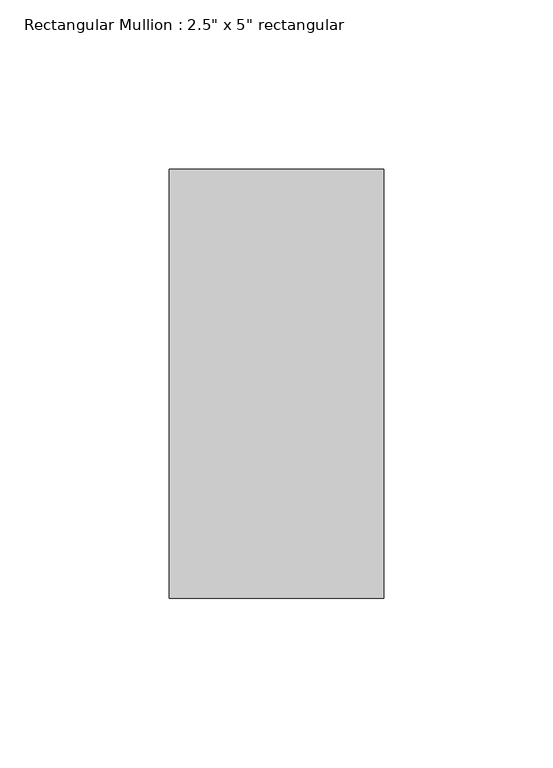
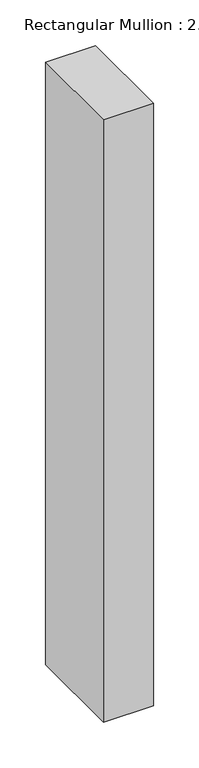
"""IFC4 building model written with IfcOpenShell, lengths in millimetres: member geometry."""

from ifc_helpers import new_model, si_unit, frame, origin, place, context, project, spatial, polyline, outline, extrude, source, transform, mapped, element, save


def member_6e893292(model_context):
    return source(origin(), model_context, "Body", "SweptSolid", [
        extrude(outline(polyline([(31.75, 63.5), (31.75, -63.5), (-31.75, -63.5), (-31.75, 63.5), (31.75, 63.5)])), frame((0.0, 0.0, -806.1882113), z_axis=(0.0, 0.0, 1.0), x_axis=(1.0, 0.0, 0.0)), (0.0, 0.0, 1.0), 806.1882113),
    ])


if __name__ == "__main__":
    model = new_model("IFC4")
    model_context = context("Model", 3, world=origin())
    ifc_project = project(units=[si_unit("LENGTHUNIT", "METRE", prefix="MILLI")], contexts=[model_context])
    site = spatial("IfcSite", under=ifc_project)
    building = spatial("IfcBuilding", under=site)
    placement = place(None, origin())
    member_shape = member_6e893292(model_context)
    element("IfcMember", 1, ObjectType="Rectangular Mullion : 2.5\" x 5\" rectangular", at=placement, inside=building, context=model_context, shape_type="MappedRepresentation", body=[
        mapped(member_shape, transform((0.0, 0.0, 0.0), x_axis=(1.0, 0.0, 0.0), y_axis=(0.0, 1.0, 0.0), z_axis=(0.0, 0.0, 1.0))),
    ])
    save(model, "model.ifc")

# Revit data of these elements
# Type "Rectangular Mullion : 2.5\" x 5\" rectangular"
#   built-in parameter 1007304 = 0.416667 (stored number, unit not read)
#   built-in parameter 1007301 = 0.104167 (stored number, unit not read)
#   built-in parameter 1007300 = 0.104167 (stored number, unit not read)
# Element 1 (IfcMember, "Rectangular Mullion : 2.5\" x 5\" rectangular")
#   Materials on its faces: "Aluminum"
# Materials
#   "Aluminum": class "Metal", colour RGB 247 247 247, transparency 0, Description = "Aluminum 6061", Cost = 0
